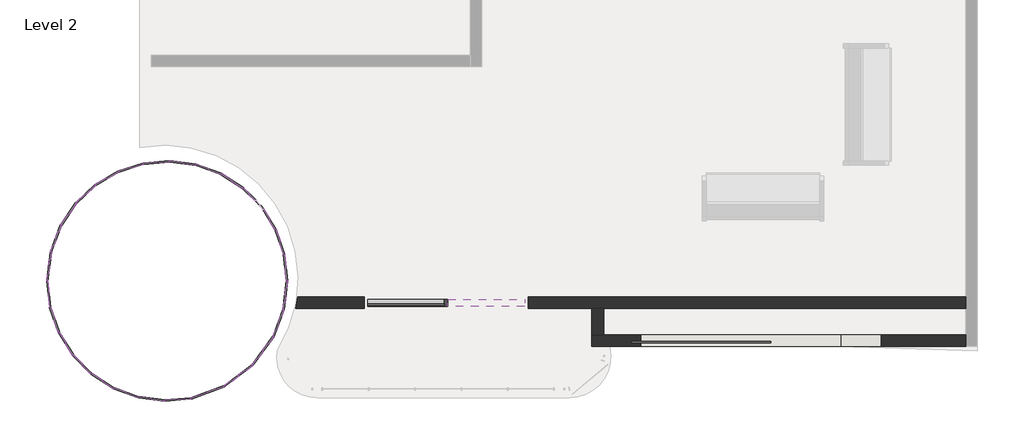
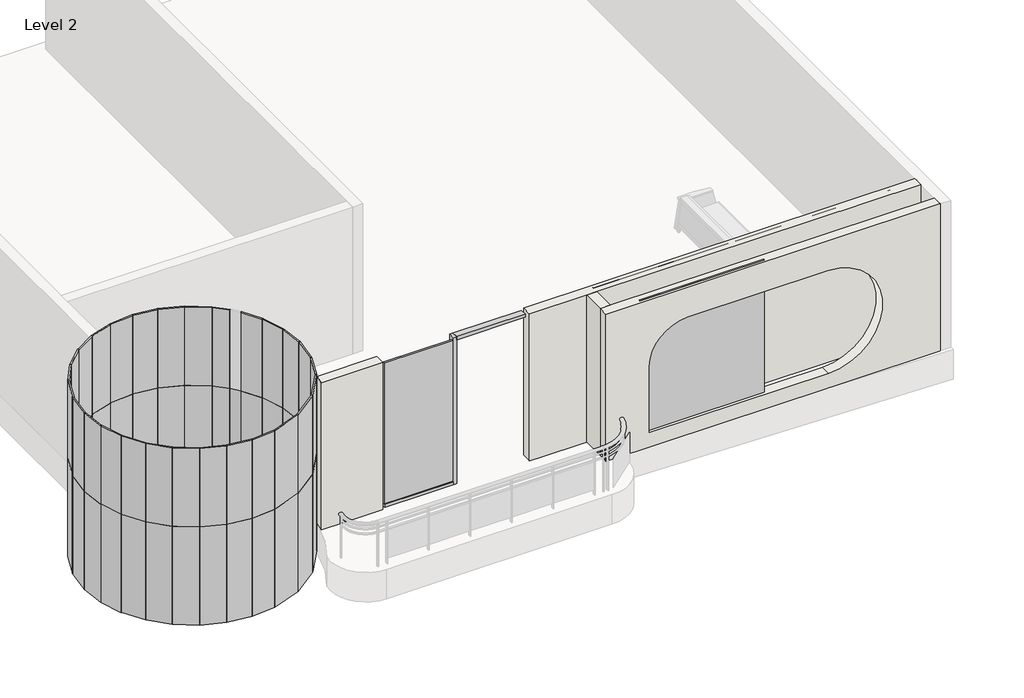
# One storey, part 1 of 2: 58 plates, 4 walls, 3 members.
"""IFC4 building model written with IfcOpenShell, lengths in millimetres."""

from ifc_helpers import new_model, si_unit, point, frame, frame_2d, origin, place, context, project, spatial, polyline, circle_curve, trimmed, segment, composite_curve, outline, extrude, faceted_brep, transform, mapped, element, save
from ifc_brep_helpers import plane_surface, revolved_surface, advanced_brep
from components import member_eaba9652, member_0c868e12, system_panel_glazed_f1c144f9, system_panel_glazed_8ed2b2ee, system_panel_glazed_c7815b78, system_panel_glazed_220ba5f3, system_panel_glazed_11fb153e, system_panel_glazed_2f540b85, system_panel_glazed_4848e608, system_panel_glazed_8b35a0ff, system_panel_glazed_6d1bb68c, system_panel_glazed_cb3ffd69, system_panel_glazed_404d015f, system_panel_glazed_7b556abe, system_panel_glazed_c60cfc80, system_panel_glazed_8d480110

model = new_model("IFC4")

# Units and contexts
model_context = context("Model", 3, world=origin())
ifc_project = project(units=[si_unit("LENGTHUNIT", "METRE", prefix="MILLI")], contexts=[model_context])

# Site, building, storey
site = spatial("IfcSite", under=ifc_project)
building = spatial("IfcBuilding", under=site)
storey = spatial("IfcBuildingStorey", under=building, Name="Level 2", Elevation=3048.0)

# Members
placement = place(None, origin())
member_shape = member_eaba9652(model_context)
element("IfcMember", 1, ObjectType="Rectangular Mullion : 2.5\" x 5\" rectangular", at=placement, inside=storey, context=model_context, shape_type="MappedRepresentation", body=[
    mapped(member_shape, transform((-7672.5789001, -1482.8937024, 3657.6), x_axis=(-1.0, 0.0, 0.0), y_axis=(0.0, 1.0, 0.0), z_axis=(0.0, 0.0, -1.0))),
])
member_2_shape = member_0c868e12(model_context)
element("IfcMember", 2, ObjectType="Rectangular Mullion : 2.5\" x 5\" rectangular", at=placement, inside=storey, context=model_context, shape_type="MappedRepresentation", body=[
    mapped(member_2_shape, transform((-7640.8289001, -1482.8937024, 6705.6), x_axis=(0.0, 0.0, 1.0), y_axis=(0.0, 1.0, 0.0), z_axis=(-1.0, 0.0, 0.0))),
])
element("IfcMember", 3, ObjectType="Rectangular Mullion : 2.5\" x 5\" rectangular", at=placement, inside=storey, context=model_context, shape_type="MappedRepresentation", body=[
    mapped(member_2_shape, transform((-7704.3289001, -1482.8937024, 3657.6), x_axis=(0.0, 0.0, -1.0), y_axis=(0.0, 1.0, 0.0), z_axis=(1.0, 0.0, 0.0))),
])

# Plates
system_panel_glazed_shape = system_panel_glazed_f1c144f9(model_context)
element("IfcPlate", 4, ObjectType="System Panel : Glazed", at=placement, inside=storey, context=model_context, shape_type="MappedRepresentation", body=[
    mapped(system_panel_glazed_shape, transform((-14541.9245022, -346.5978939, 3657.6), x_axis=(-0.3551689475306269, -0.9348021281051873, 0.0), y_axis=(0.9348021281051873, -0.3551689475306269, 0.0), z_axis=(0.0, 0.0, 1.0))),
])
element("IfcPlate", 5, ObjectType="System Panel : Glazed", at=placement, inside=storey, context=model_context, shape_type="MappedRepresentation", body=[
    mapped(system_panel_glazed_shape, transform((-10582.1178502, -1851.0877948, 3657.6), x_axis=(0.35516894753064066, 0.934802128105182, 0.0), y_axis=(-0.934802128105182, 0.35516894753064066, 0.0), z_axis=(0.0, 0.0, 1.0))),
])
element("IfcPlate", 6, ObjectType="System Panel : Glazed", at=placement, inside=storey, context=model_context, shape_type="MappedRepresentation", body=[
    mapped(system_panel_glazed_shape, transform((-10459.5232171, -1354.5613954, 3657.6), x_axis=(0.12073632210407238, 0.9926846128175765, 0.0), y_axis=(-0.9926846128175765, 0.12073632210407238, 0.0), z_axis=(0.0, 0.0, 1.0))),
])
element("IfcPlate", 7, ObjectType="System Panel : Glazed", at=placement, inside=storey, context=model_context, shape_type="MappedRepresentation", body=[
    mapped(system_panel_glazed_shape, transform((-14664.5191354, -843.1242933, 3657.6), x_axis=(-0.12073632210406242, -0.9926846128175777, 0.0), y_axis=(0.9926846128175777, -0.12073632210406242, 0.0), z_axis=(0.0, 0.0, 1.0))),
])
system_panel_glazed_2_shape = system_panel_glazed_8ed2b2ee(model_context)
element("IfcPlate", 8, ObjectType="System Panel : Glazed", at=placement, inside=storey, context=model_context, shape_type="MappedRepresentation", body=[
    mapped(system_panel_glazed_2_shape, transform((-11841.3777431, -3082.3793017, 3657.6), x_axis=(0.9398911711666007, 0.34147413718036645, 0.0), y_axis=(-0.34147413718036645, 0.9398911711666007, 0.0), z_axis=(0.0, 0.0, 1.0))),
])
element("IfcPlate", 9, ObjectType="System Panel : Glazed", at=placement, inside=storey, context=model_context, shape_type="MappedRepresentation", body=[
    mapped(system_panel_glazed_2_shape, transform((-10858.9635423, -2345.1728692, 3657.6), x_axis=(0.5905687200141164, 0.8069873524045393, 0.0), y_axis=(-0.8069873524045393, 0.5905687200141164, 0.0), z_axis=(0.0, 0.0, 1.0))),
])
element("IfcPlate", 10, ObjectType="System Panel : Glazed", at=placement, inside=storey, context=model_context, shape_type="MappedRepresentation", body=[
    mapped(system_panel_glazed_2_shape, transform((-11295.3522982, -2786.8279712, 3657.6), x_axis=(0.7998453025525061, 0.6002062078858317, 0.0), y_axis=(-0.6002062078858317, 0.7998453025525061, 0.0), z_axis=(0.0, 0.0, 1.0))),
])
system_panel_glazed_3_shape = system_panel_glazed_c7815b78(model_context)
element("IfcPlate", 11, ObjectType="System Panel : Glazed", at=placement, inside=storey, context=model_context, shape_type="MappedRepresentation", body=[
    mapped(system_panel_glazed_3_shape, transform((-10454.4737362, -864.5204039, 3657.6), x_axis=(-0.11050163420416613, 0.993875942378227, 0.0), y_axis=(-0.993875942378227, -0.11050163420416613, 0.0), z_axis=(0.0, 0.0, 1.0))),
])
element("IfcPlate", 12, ObjectType="System Panel : Glazed", at=placement, inside=storey, context=model_context, shape_type="MappedRepresentation", body=[
    mapped(system_panel_glazed_3_shape, transform((-14669.5686163, -1333.1652848, 3657.6), x_axis=(0.11050163420415138, -0.9938759423782286, 0.0), y_axis=(0.9938759423782286, 0.11050163420415138, 0.0), z_axis=(0.0, 0.0, 1.0))),
])
element("IfcPlate", 13, ObjectType="System Panel : Glazed", at=placement, inside=storey, context=model_context, shape_type="MappedRepresentation", body=[
    mapped(system_panel_glazed_3_shape, transform((-11410.1424167, 681.5611944, 3657.6), x_axis=(-0.8396018558176894, 0.5432022861766066, 0.0), y_axis=(-0.5432022861766066, -0.8396018558176894, 0.0), z_axis=(0.0, 0.0, 1.0))),
])
element("IfcPlate", 14, ObjectType="System Panel : Glazed", at=placement, inside=storey, context=model_context, shape_type="MappedRepresentation", body=[
    mapped(system_panel_glazed_3_shape, transform((-13212.0893695, 919.590846, 3657.6), x_axis=(-0.9518517343814786, -0.3065587639506839, 0.0), y_axis=(0.3065587639506839, -0.9518517343814786, 0.0), z_axis=(0.0, 0.0, 1.0))),
])
element("IfcPlate", 15, ObjectType="System Panel : Glazed", at=placement, inside=storey, context=model_context, shape_type="MappedRepresentation", body=[
    mapped(system_panel_glazed_3_shape, transform((-12839.7224363, -3201.1142893, 3657.6), x_axis=(0.9913878918151698, -0.1309581916577702, 0.0), y_axis=(0.1309581916577702, 0.9913878918151698, 0.0), z_axis=(0.0, 0.0, 1.0))),
])
element("IfcPlate", 16, ObjectType="System Panel : Glazed", at=placement, inside=storey, context=model_context, shape_type="MappedRepresentation", body=[
    mapped(system_panel_glazed_3_shape, transform((-14365.783041, -2213.7896382, 3657.6), x_axis=(0.5257859322352114, -0.8506169252157811, 0.0), y_axis=(0.8506169252157811, 0.5257859322352114, 0.0), z_axis=(0.0, 0.0, 1.0))),
])
element("IfcPlate", 17, ObjectType="System Panel : Glazed", at=placement, inside=storey, context=model_context, shape_type="MappedRepresentation", body=[
    mapped(system_panel_glazed_3_shape, transform((-13713.8999358, -2879.2468831, 3657.6), x_axis=(0.8396018558176805, -0.5432022861766201, 0.0), y_axis=(0.5432022861766201, 0.8396018558176805, 0.0), z_axis=(0.0, 0.0, 1.0))),
])
element("IfcPlate", 18, ObjectType="System Panel : Glazed", at=placement, inside=storey, context=model_context, shape_type="MappedRepresentation", body=[
    mapped(system_panel_glazed_3_shape, transform((-14014.4059364, 446.2272921, 3657.6), x_axis=(-0.7286232370002992, -0.6849147235263715, 0.0), y_axis=(0.6849147235263715, -0.7286232370002992, 0.0), z_axis=(0.0, 0.0, 1.0))),
])
element("IfcPlate", 19, ObjectType="System Panel : Glazed", at=placement, inside=storey, context=model_context, shape_type="MappedRepresentation", body=[
    mapped(system_panel_glazed_3_shape, transform((-12284.3199161, 1003.4286006, 3657.6), x_axis=(-0.9913878918151723, 0.1309581916577514, 0.0), y_axis=(-0.1309581916577514, -0.9913878918151723, 0.0), z_axis=(0.0, 0.0, 1.0))),
])
element("IfcPlate", 20, ObjectType="System Panel : Glazed", at=placement, inside=storey, context=model_context, shape_type="MappedRepresentation", body=[
    mapped(system_panel_glazed_3_shape, transform((-12752.8652893, 1013.0855973, 3657.6), x_axis=(-0.9959419324521102, -0.08999815100076568, 0.0), y_axis=(0.08999815100076568, -0.9959419324521102, 0.0), z_axis=(0.0, 0.0, 1.0))),
])
element("IfcPlate", 21, ObjectType="System Panel : Glazed", at=placement, inside=storey, context=model_context, shape_type="MappedRepresentation", body=[
    mapped(system_panel_glazed_3_shape, transform((-11829.3381514, 891.0915272, 3657.6), x_axis=(-0.9384120429483949, 0.34551821608913763, 0.0), y_axis=(-0.34551821608913763, -0.9384120429483949, 0.0), z_axis=(0.0, 0.0, 1.0))),
])
element("IfcPlate", 22, ObjectType="System Panel : Glazed", at=placement, inside=storey, context=model_context, shape_type="MappedRepresentation", body=[
    mapped(system_panel_glazed_3_shape, transform((-10557.4115054, -407.3204039, 3657.6), x_axis=(-0.3261077326604367, 0.9453326116764772, 0.0), y_axis=(-0.9453326116764772, -0.3261077326604367, 0.0), z_axis=(0.0, 0.0, 1.0))),
])
element("IfcPlate", 23, ObjectType="System Panel : Glazed", at=placement, inside=storey, context=model_context, shape_type="MappedRepresentation", body=[
    mapped(system_panel_glazed_3_shape, transform((-12371.1770631, -3210.771286, 3657.6), x_axis=(0.9959419324521115, 0.08999815100075, 0.0), y_axis=(-0.08999815100075, 0.9959419324521115, 0.0), z_axis=(0.0, 0.0, 1.0))),
])
element("IfcPlate", 24, ObjectType="System Panel : Glazed", at=placement, inside=storey, context=model_context, shape_type="MappedRepresentation", body=[
    mapped(system_panel_glazed_3_shape, transform((-13294.7042011, -3088.7772159, 3657.6), x_axis=(0.9384120429483891, -0.34551821608915334, 0.0), y_axis=(0.34551821608915334, 0.9384120429483891, 0.0), z_axis=(0.0, 0.0, 1.0))),
])
element("IfcPlate", 25, ObjectType="System Panel : Glazed", at=placement, inside=storey, context=model_context, shape_type="MappedRepresentation", body=[
    mapped(system_panel_glazed_3_shape, transform((-14076.8350959, -2582.7572647, 3657.6), x_axis=(0.6997834615185511, -0.7143550286692988, 0.0), y_axis=(0.7143550286692988, 0.6997834615185511, 0.0), z_axis=(0.0, 0.0, 1.0))),
])
element("IfcPlate", 26, ObjectType="System Panel : Glazed", at=placement, inside=storey, context=model_context, shape_type="MappedRepresentation", body=[
    mapped(system_panel_glazed_3_shape, transform((-14566.6308471, -1790.3652848, 3657.6), x_axis=(0.32610773266042153, -0.9453326116764824, 0.0), y_axis=(0.9453326116764824, 0.32610773266042153, 0.0), z_axis=(0.0, 0.0, 1.0))),
])
element("IfcPlate", 27, ObjectType="System Panel : Glazed", at=placement, inside=storey, context=model_context, shape_type="MappedRepresentation", body=[
    mapped(system_panel_glazed_3_shape, transform((-14318.3113206, 89.4787227, 3657.6), x_axis=(-0.5603879632167612, -0.8282302401396425, 0.0), y_axis=(0.8282302401396425, -0.5603879632167612, 0.0), z_axis=(0.0, 0.0, 1.0))),
])
element("IfcPlate", 28, ObjectType="System Panel : Glazed", at=placement, inside=storey, context=model_context, shape_type="MappedRepresentation", body=[
    mapped(system_panel_glazed_3_shape, transform((-13639.5625299, 727.5108588, 3657.6), x_axis=(-0.8612707706620223, -0.508146297441245, 0.0), y_axis=(0.508146297441245, -0.8612707706620223, 0.0), z_axis=(0.0, 0.0, 1.0))),
])
system_panel_glazed_4_shape = system_panel_glazed_220ba5f3(model_context)
element("IfcPlate", 29, ObjectType="System Panel : Glazed", at=placement, inside=storey, context=model_context, shape_type="MappedRepresentation", body=[
    mapped(system_panel_glazed_4_shape, transform((-10742.3305673, -4.7597883, 3657.6), x_axis=(-0.5152811917631037, 0.8570211744263939, 0.0), y_axis=(-0.8570211744263939, -0.5152811917631037, 0.0), z_axis=(0.0, 0.0, 1.0))),
])
system_panel_glazed_5_shape = system_panel_glazed_11fb153e(model_context)
element("IfcPlate", 30, ObjectType="System Panel : Glazed", at=placement, inside=storey, context=model_context, shape_type="MappedRepresentation", body=[
    mapped(system_panel_glazed_5_shape, transform((-11098.0043985, 445.2241463, 3657.6), x_axis=(-0.7256671855033587, 0.6880458821064435, 0.0), y_axis=(-0.6880458821064435, -0.7256671855033587, 0.0), z_axis=(0.0, 0.0, 1.0))),
])
system_panel_glazed_6_shape = system_panel_glazed_2f540b85(model_context)
element("IfcPlate", 31, ObjectType="System Panel : Glazed", at=placement, inside=storey, context=model_context, shape_type="MappedRepresentation", body=[
    mapped(system_panel_glazed_6_shape, transform((-10917.0903061, 255.9395759, 3657.6), x_axis=(-0.6357445726375757, 0.7718995001694627, 0.0), y_axis=(-0.7718995001694627, -0.6357445726375757, 0.0), z_axis=(0.0, 0.0, 1.0))),
])
system_panel_glazed_7_shape = system_panel_glazed_4848e608(model_context)
element("IfcPlate", 32, ObjectType="System Panel : Glazed", at=placement, inside=storey, context=model_context, shape_type="MappedRepresentation", body=[
    mapped(system_panel_glazed_7_shape, transform((-14669.5686163, -1333.1652848, 5689.6), x_axis=(0.11050163420415138, -0.9938759423782286, 0.0), y_axis=(0.9938759423782286, 0.11050163420415138, 0.0), z_axis=(0.0, 0.0, 1.0))),
])
element("IfcPlate", 33, ObjectType="System Panel : Glazed", at=placement, inside=storey, context=model_context, shape_type="MappedRepresentation", body=[
    mapped(system_panel_glazed_7_shape, transform((-14365.783041, -2213.7896382, 5689.6), x_axis=(0.5257859322352114, -0.8506169252157811, 0.0), y_axis=(0.8506169252157811, 0.5257859322352114, 0.0), z_axis=(0.0, 0.0, 1.0))),
])
element("IfcPlate", 34, ObjectType="System Panel : Glazed", at=placement, inside=storey, context=model_context, shape_type="MappedRepresentation", body=[
    mapped(system_panel_glazed_7_shape, transform((-13713.8999358, -2879.2468831, 5689.6), x_axis=(0.8396018558176805, -0.5432022861766201, 0.0), y_axis=(0.5432022861766201, 0.8396018558176805, 0.0), z_axis=(0.0, 0.0, 1.0))),
])
element("IfcPlate", 35, ObjectType="System Panel : Glazed", at=placement, inside=storey, context=model_context, shape_type="MappedRepresentation", body=[
    mapped(system_panel_glazed_7_shape, transform((-12839.7224363, -3201.1142893, 5689.6), x_axis=(0.9913878918151698, -0.13095819165777017, 0.0), y_axis=(0.13095819165777017, 0.9913878918151698, 0.0), z_axis=(0.0, 0.0, 1.0))),
])
element("IfcPlate", 36, ObjectType="System Panel : Glazed", at=placement, inside=storey, context=model_context, shape_type="MappedRepresentation", body=[
    mapped(system_panel_glazed_7_shape, transform((-12371.1770631, -3210.771286, 5689.6), x_axis=(0.9959419324521115, 0.08999815100075002, 0.0), y_axis=(-0.08999815100075002, 0.9959419324521115, 0.0), z_axis=(0.0, 0.0, 1.0))),
])
element("IfcPlate", 37, ObjectType="System Panel : Glazed", at=placement, inside=storey, context=model_context, shape_type="MappedRepresentation", body=[
    mapped(system_panel_glazed_7_shape, transform((-13294.7042011, -3088.7772159, 5689.6), x_axis=(0.9384120429483891, -0.34551821608915334, 0.0), y_axis=(0.34551821608915334, 0.9384120429483891, 0.0), z_axis=(0.0, 0.0, 1.0))),
])
element("IfcPlate", 38, ObjectType="System Panel : Glazed", at=placement, inside=storey, context=model_context, shape_type="MappedRepresentation", body=[
    mapped(system_panel_glazed_7_shape, transform((-14076.8350959, -2582.7572647, 5689.6), x_axis=(0.6997834615185511, -0.7143550286692988, 0.0), y_axis=(0.7143550286692988, 0.6997834615185511, 0.0), z_axis=(0.0, 0.0, 1.0))),
])
element("IfcPlate", 39, ObjectType="System Panel : Glazed", at=placement, inside=storey, context=model_context, shape_type="MappedRepresentation", body=[
    mapped(system_panel_glazed_7_shape, transform((-14566.6308471, -1790.3652848, 5689.6), x_axis=(0.32610773266042153, -0.9453326116764824, 0.0), y_axis=(0.9453326116764824, 0.32610773266042153, 0.0), z_axis=(0.0, 0.0, 1.0))),
])
element("IfcPlate", 40, ObjectType="System Panel : Glazed", at=placement, inside=storey, context=model_context, shape_type="MappedRepresentation", body=[
    mapped(system_panel_glazed_7_shape, transform((-10454.4737362, -864.5204039, 5689.6), x_axis=(-0.11050163420416614, 0.993875942378227, 0.0), y_axis=(-0.993875942378227, -0.11050163420416614, 0.0), z_axis=(0.0, 0.0, 1.0))),
])
element("IfcPlate", 41, ObjectType="System Panel : Glazed", at=placement, inside=storey, context=model_context, shape_type="MappedRepresentation", body=[
    mapped(system_panel_glazed_7_shape, transform((-10557.4115054, -407.3204039, 5689.6), x_axis=(-0.32610773266043674, 0.9453326116764772, 0.0), y_axis=(-0.9453326116764772, -0.32610773266043674, 0.0), z_axis=(0.0, 0.0, 1.0))),
])
element("IfcPlate", 42, ObjectType="System Panel : Glazed", at=placement, inside=storey, context=model_context, shape_type="MappedRepresentation", body=[
    mapped(system_panel_glazed_7_shape, transform((-11410.1424167, 681.5611944, 5689.6), x_axis=(-0.8396018558176894, 0.5432022861766066, 0.0), y_axis=(-0.5432022861766066, -0.8396018558176894, 0.0), z_axis=(0.0, 0.0, 1.0))),
])
element("IfcPlate", 43, ObjectType="System Panel : Glazed", at=placement, inside=storey, context=model_context, shape_type="MappedRepresentation", body=[
    mapped(system_panel_glazed_7_shape, transform((-11829.3381514, 891.0915272, 5689.6), x_axis=(-0.9384120429483949, 0.34551821608913763, 0.0), y_axis=(-0.34551821608913763, -0.9384120429483949, 0.0), z_axis=(0.0, 0.0, 1.0))),
])
element("IfcPlate", 44, ObjectType="System Panel : Glazed", at=placement, inside=storey, context=model_context, shape_type="MappedRepresentation", body=[
    mapped(system_panel_glazed_7_shape, transform((-12284.3199161, 1003.4286006, 5689.6), x_axis=(-0.9913878918151723, 0.13095819165775144, 0.0), y_axis=(-0.13095819165775144, -0.9913878918151723, 0.0), z_axis=(0.0, 0.0, 1.0))),
])
element("IfcPlate", 45, ObjectType="System Panel : Glazed", at=placement, inside=storey, context=model_context, shape_type="MappedRepresentation", body=[
    mapped(system_panel_glazed_7_shape, transform((-12752.8652893, 1013.0855973, 5689.6), x_axis=(-0.9959419324521102, -0.08999815100076569, 0.0), y_axis=(0.08999815100076569, -0.9959419324521102, 0.0), z_axis=(0.0, 0.0, 1.0))),
])
element("IfcPlate", 46, ObjectType="System Panel : Glazed", at=placement, inside=storey, context=model_context, shape_type="MappedRepresentation", body=[
    mapped(system_panel_glazed_7_shape, transform((-13212.0893695, 919.590846, 5689.6), x_axis=(-0.9518517343814786, -0.3065587639506839, 0.0), y_axis=(0.3065587639506839, -0.9518517343814786, 0.0), z_axis=(0.0, 0.0, 1.0))),
])
element("IfcPlate", 47, ObjectType="System Panel : Glazed", at=placement, inside=storey, context=model_context, shape_type="MappedRepresentation", body=[
    mapped(system_panel_glazed_7_shape, transform((-13639.5625299, 727.5108588, 5689.6), x_axis=(-0.8612707706620224, -0.5081462974412448, 0.0), y_axis=(0.5081462974412448, -0.8612707706620224, 0.0), z_axis=(0.0, 0.0, 1.0))),
])
element("IfcPlate", 48, ObjectType="System Panel : Glazed", at=placement, inside=storey, context=model_context, shape_type="MappedRepresentation", body=[
    mapped(system_panel_glazed_7_shape, transform((-14014.4059364, 446.2272921, 5689.6), x_axis=(-0.7286232370002992, -0.6849147235263715, 0.0), y_axis=(0.6849147235263715, -0.7286232370002992, 0.0), z_axis=(0.0, 0.0, 1.0))),
])
element("IfcPlate", 49, ObjectType="System Panel : Glazed", at=placement, inside=storey, context=model_context, shape_type="MappedRepresentation", body=[
    mapped(system_panel_glazed_7_shape, transform((-14318.3113206, 89.4787227, 5689.6), x_axis=(-0.5603879632167612, -0.8282302401396425, 0.0), y_axis=(0.8282302401396425, -0.5603879632167612, 0.0), z_axis=(0.0, 0.0, 1.0))),
])
system_panel_glazed_8_shape = system_panel_glazed_8b35a0ff(model_context)
element("IfcPlate", 50, ObjectType="System Panel : Glazed", at=placement, inside=storey, context=model_context, shape_type="MappedRepresentation", body=[
    mapped(system_panel_glazed_8_shape, transform((-10742.3305673, -4.7597883, 5689.6), x_axis=(-0.5152811917631037, 0.8570211744263939, 0.0), y_axis=(-0.8570211744263939, -0.5152811917631037, 0.0), z_axis=(0.0, 0.0, 1.0))),
])
system_panel_glazed_9_shape = system_panel_glazed_6d1bb68c(model_context)
element("IfcPlate", 51, ObjectType="System Panel : Glazed", at=placement, inside=storey, context=model_context, shape_type="MappedRepresentation", body=[
    mapped(system_panel_glazed_9_shape, transform((-11098.0043985, 445.2241463, 5689.6), x_axis=(-0.7256671855033587, 0.6880458821064435, 0.0), y_axis=(-0.6880458821064435, -0.7256671855033587, 0.0), z_axis=(0.0, 0.0, 1.0))),
])
system_panel_glazed_10_shape = system_panel_glazed_cb3ffd69(model_context)
element("IfcPlate", 52, ObjectType="System Panel : Glazed", at=placement, inside=storey, context=model_context, shape_type="MappedRepresentation", body=[
    mapped(system_panel_glazed_10_shape, transform((-10582.1178502, -1851.0877948, 5689.6), x_axis=(0.3551689475306406, 0.934802128105182, 0.0), y_axis=(-0.934802128105182, 0.3551689475306406, 0.0), z_axis=(0.0, 0.0, 1.0))),
])
element("IfcPlate", 53, ObjectType="System Panel : Glazed", at=placement, inside=storey, context=model_context, shape_type="MappedRepresentation", body=[
    mapped(system_panel_glazed_10_shape, transform((-10459.5232171, -1354.5613954, 5689.6), x_axis=(0.12073632210407237, 0.9926846128175765, 0.0), y_axis=(-0.9926846128175765, 0.12073632210407237, 0.0), z_axis=(0.0, 0.0, 1.0))),
])
element("IfcPlate", 54, ObjectType="System Panel : Glazed", at=placement, inside=storey, context=model_context, shape_type="MappedRepresentation", body=[
    mapped(system_panel_glazed_10_shape, transform((-14541.9245022, -346.5978939, 5689.6), x_axis=(-0.35516894753062683, -0.9348021281051873, 0.0), y_axis=(0.9348021281051873, -0.35516894753062683, 0.0), z_axis=(0.0, 0.0, 1.0))),
])
element("IfcPlate", 55, ObjectType="System Panel : Glazed", at=placement, inside=storey, context=model_context, shape_type="MappedRepresentation", body=[
    mapped(system_panel_glazed_10_shape, transform((-14664.5191354, -843.1242933, 5689.6), x_axis=(-0.12073632210406242, -0.9926846128175777, 0.0), y_axis=(0.9926846128175777, -0.12073632210406242, 0.0), z_axis=(0.0, 0.0, 1.0))),
])
system_panel_glazed_11_shape = system_panel_glazed_404d015f(model_context)
element("IfcPlate", 56, ObjectType="System Panel : Glazed", at=placement, inside=storey, context=model_context, shape_type="MappedRepresentation", body=[
    mapped(system_panel_glazed_11_shape, transform((-11841.3777431, -3082.3793017, 5689.6), x_axis=(0.9398911711666007, 0.34147413718036645, 0.0), y_axis=(-0.34147413718036645, 0.9398911711666007, 0.0), z_axis=(0.0, 0.0, 1.0))),
])
element("IfcPlate", 57, ObjectType="System Panel : Glazed", at=placement, inside=storey, context=model_context, shape_type="MappedRepresentation", body=[
    mapped(system_panel_glazed_11_shape, transform((-10858.9635423, -2345.1728692, 5689.6), x_axis=(0.5905687200141164, 0.8069873524045393, 0.0), y_axis=(-0.8069873524045393, 0.5905687200141164, 0.0), z_axis=(0.0, 0.0, 1.0))),
])
element("IfcPlate", 58, ObjectType="System Panel : Glazed", at=placement, inside=storey, context=model_context, shape_type="MappedRepresentation", body=[
    mapped(system_panel_glazed_11_shape, transform((-11295.3522982, -2786.8279712, 5689.6), x_axis=(0.7998453025525061, 0.6002062078858317, 0.0), y_axis=(-0.6002062078858317, 0.7998453025525061, 0.0), z_axis=(0.0, 0.0, 1.0))),
])
system_panel_glazed_12_shape = system_panel_glazed_7b556abe(model_context)
element("IfcPlate", 59, ObjectType="System Panel : Glazed", at=placement, inside=storey, context=model_context, shape_type="MappedRepresentation", body=[
    mapped(system_panel_glazed_12_shape, transform((-8376.2702257, -1482.8937024, 3721.1), x_axis=(-1.0, 0.0, 0.0), y_axis=(0.0, -1.0, 0.0), z_axis=(0.0, 0.0, 1.0))),
])
system_panel_glazed_13_shape = system_panel_glazed_c60cfc80(model_context)
element("IfcPlate", 60, ObjectType="System Panel : Glazed", at=placement, inside=storey, context=model_context, shape_type="MappedRepresentation", body=[
    mapped(system_panel_glazed_13_shape, transform((-3198.1462491, -2143.2937024, 3657.6), x_axis=(-1.0, 0.0, 0.0), y_axis=(0.0, -1.0, 0.0), z_axis=(0.0, 0.0, 1.0))),
])
system_panel_glazed_14_shape = system_panel_glazed_8d480110(model_context)
element("IfcPlate", 61, ObjectType="System Panel : Glazed", at=placement, inside=storey, context=model_context, shape_type="MappedRepresentation", body=[
    mapped(system_panel_glazed_14_shape, transform((-1737.6462491, -1482.8937024, 3657.6), x_axis=(1.0, 0.0, 0.0), y_axis=(0.0, 1.0, 0.0), z_axis=(0.0, 0.0, 1.0))),
])

# Walls
element("IfcWall", 62, ObjectType="Generic - 8\"", at=placement, inside=storey, context=model_context, shape_type="SweptSolid", body=[
    extrude(outline(composite_curve([segment(polyline([(-9111.7115512, -1584.4937024), (-10312.8376694, -1584.4937024)]), True, "CONTINUOUS"), segment(trimmed(circle_curve(frame_2d((-12612.6150686, -1075.1054509)), 2355.5153315), [point((-10312.8376694, -1584.4937024))], [point((-10277.0848865, -1381.2937024))], True, "CARTESIAN"), True, "CONTINUOUS"), segment(polyline([(-10277.0848865, -1381.2937024), (-9111.7115512, -1381.2937024), (-9111.7115512, -1584.4937024)]), True, "CONTINUOUS")], self_intersect=False)), frame((0.0, 0.0, 3657.6), z_axis=(0.0, 0.0, 1.0), x_axis=(1.0, 0.0, 0.0)), (0.0, 0.0, 1.0), 3048.0),
])
element("IfcWall", 63, ObjectType="Generic - 8\"", at=placement, inside=storey, context=model_context, shape_type="AdvancedBrep", body=[
    advanced_brep(
    [(1437.3537509, -2041.6937024, 3657.6), (-4912.6462491, -2041.6937024, 3657.6), (-5115.8462491, -2041.6937024, 3657.6), (-5115.8462491, -2041.6937024, 6705.6), (-4912.6462491, -2041.6937024, 6705.6), (1437.3537509, -2041.6937024, 6705.6), (-4264.9683746, -2041.6937024, 5334.0), (-4264.9683746, -2041.6937024, 3962.4), (-759.7683746, -2041.6937024, 3962.4), (-759.7683746, -2041.6937024, 6088.3415142), (-3510.6268604, -2041.6937024, 6088.3415142), (1437.3537509, -2244.8937024, 3657.6), (1437.3537509, -2244.8937024, 6705.6), (-5115.8462491, -2244.8937024, 6705.6), (-5115.8462491, -2244.8937024, 3657.6), (-4264.9683746, -2244.8937024, 5334.0), (-3510.6268604, -2244.8937024, 6088.3415142), (-759.7683746, -2244.8937024, 6088.3415142), (-759.7683746, -2244.8937024, 3962.4), (-4264.9683746, -2244.8937024, 3962.4)],
    [
        (0, 1),
        (1, 2),
        (2, 3),
        (3, 4),
        (4, 5),
        (5, 0),
        (6, 7),
        (7, 8),
        (8, 9, circle_curve(frame((-759.7683746, -2041.6937024, 5025.3707571), z_axis=(0.0, -1.0, 0.0), x_axis=(1.0, 0.0, 0.0)), 1062.9707571)),
        (9, 10),
        (10, 6, circle_curve(frame((-3510.6268604, -2041.6937024, 5334.0), z_axis=(0.0, -1.0, 0.0), x_axis=(1.0, 0.0, 0.0)), 754.3415142)),
        (11, 12),
        (12, 13),
        (13, 14),
        (14, 11),
        (15, 16, circle_curve(frame((-3510.6268604, -2244.8937024, 5334.0), z_axis=(0.0, 1.0, 0.0), x_axis=(1.0, 0.0, 0.0)), 754.3415142)),
        (16, 17),
        (17, 18, circle_curve(frame((-759.7683746, -2244.8937024, 5025.3707571), z_axis=(0.0, 1.0, 0.0), x_axis=(1.0, 0.0, 0.0)), 1062.9707571)),
        (18, 19),
        (19, 15),
        (2, 14),
        (13, 3),
        (5, 12),
        (11, 0),
        (6, 15),
        (19, 7),
        (18, 8),
        (17, 9),
        (16, 10),
    ],
    [
        plane_surface(frame((1538.9537509, -2041.6937024, 3657.6), z_axis=(0.0, 1.0, 0.0), x_axis=(-1.0, 0.0, 0.0))),
        plane_surface(frame((1538.9537509, -2244.8937024, 3657.6), z_axis=(0.0, -1.0, 0.0), x_axis=(1.0, 0.0, 0.0))),
        plane_surface(frame((-5115.8462491, -1482.8937024, 3657.6), z_axis=(-1.0, 0.0, 0.0), x_axis=(0.0, -1.0, 0.0))),
        plane_surface(frame((1437.3537509, 16068.5062976, 3657.6), z_axis=(1.0, 0.0, 0.0), x_axis=(0.0, -1.0, 0.0))),
        plane_surface(frame((1538.9537509, -2041.6937024, 3657.6), z_axis=(0.0, 0.0, -1.0), x_axis=(0.0, -1.0, 0.0))),
        plane_surface(frame((-5014.2462491, -2041.6937024, 6705.6), z_axis=(0.0, 0.0, 1.0), x_axis=(0.0, -1.0, 0.0))),
        plane_surface(frame((-4264.9683746, -2041.6937024, 5334.0), z_axis=(1.0, 0.0, 0.0), x_axis=(0.0, -1.0, 0.0))),
        plane_surface(frame((-4264.9683746, -2041.6937024, 3962.4), z_axis=(0.0, 0.0, 1.0), x_axis=(0.0, -1.0, 0.0))),
        revolved_surface(polyline([(303.2023824999999, -2244.8937024, 5025.3707571), (303.2023824999999, -2041.6937024, 5025.3707571)]), (-759.7683746, -2143.2937024, 5025.3707571), (0.0, -1.0, 0.0)),
        plane_surface(frame((-759.7683746, -2041.6937024, 6088.3415142), z_axis=(0.0, 0.0, -1.0), x_axis=(0.0, -1.0, 0.0))),
        revolved_surface(polyline([(-2756.2853462000003, -2244.8937024, 5334.0), (-2756.2853462000003, -2041.6937024, 5334.0)]), (-3510.6268604, -2143.2937024, 5334.0), (0.0, -1.0, 0.0)),
    ],
    [
        (0, [[1, 2, 3, 4, 5, 6], [7, 8, 9, 10, 11]]),
        (1, [[12, 13, 14, 15], [16, 17, 18, 19, 20]]),
        (2, [[-3, 21, -14, 22]]),
        (3, [[-6, 23, -12, 24]]),
        (4, [[-2, -1, -24, -15, -21]]),
        (5, [[-5, -4, -22, -13, -23]]),
        (6, [[-7, 25, -20, 26]]),
        (7, [[-8, -26, -19, 27]]),
        (8, [[-9, -27, -18, 28]]),
        (9, [[-10, -28, -17, 29]]),
        (10, [[-11, -29, -16, -25]]),
    ],
),
])
element("IfcWall", 64, ObjectType="Generic - 8\"", at=placement, inside=storey, context=model_context, shape_type="Brep", body=[
    faceted_brep([(-6233.4462491, -1584.4937024, 3657.6), (-5115.8462491, -1584.4937024, 3657.6), (-4912.6462491, -1584.4937024, 3657.6), (1437.3537509, -1584.4937024, 3657.6), (1437.3537509, -1584.4937024, 6705.6), (-4912.6462491, -1584.4937024, 6705.6), (-5115.8462491, -1584.4937024, 6705.6), (-6233.4462491, -1584.4937024, 6705.6), (-6233.4462491, -1381.2937024, 3657.6), (-6233.4462491, -1381.2937024, 6705.6), (1437.3537509, -1381.2937024, 6705.6), (1437.3537509, -1381.2937024, 3657.6)], [[[0, 1, 2, 3, 4, 5, 6, 7]], [[8, 9, 10, 11]], [[3, 2, 1, 0, 8, 11]], [[7, 6, 5, 4, 10, 9]], [[0, 7, 9, 8]], [[4, 3, 11, 10]]]),
])
element("IfcWall", 65, ObjectType="Generic - 8\"", at=placement, inside=storey, context=model_context, shape_type="SweptSolid", body=[
    extrude(outline(polyline([(-5115.8462491, -2041.6937024), (-5115.8462491, -1584.4937024), (-4912.6462491, -1584.4937024), (-4912.6462491, -2041.6937024), (-5115.8462491, -2041.6937024)])), frame((0.0, 0.0, 3657.6), z_axis=(0.0, 0.0, 1.0), x_axis=(1.0, 0.0, 0.0)), (0.0, 0.0, 1.0), 3048.0),
])

save(model, "model.ifc")

# Revit data of these elements
# Type "Rectangular Mullion : 2.5\" x 5\" rectangular"
#   built-in parameter 1007304 = 0.416667 (stored number, unit not read)
#   built-in parameter 1007301 = 0.104167 (stored number, unit not read)
#   built-in parameter 1007300 = 0.104167 (stored number, unit not read)
# Type "System Panel : Glazed"
#   Construction Type Id = "GSP4R"
#   Analytic Construction = "1/8 in Pilkington single glazing"
#   Visual Light Transmittance = 0.9
#   Solar Heat Gain Coefficient = 0.86
#   Heat Transfer Coefficient (U) = 1.18115 BTU/(h·ft²·°F)
# Type "Generic - 8\""
#   Assembly Code = "B2010"
#   Layers, outside or top first: 0' - 8" no material (function 1)
# Elements 1, 2, 3 (IfcMember, "Rectangular Mullion : 2.5\" x 5\" rectangular")
#   Phase Created = New Construction
#   Materials on its faces: "Iron, Ductile"
# Elements 4, 5, 6, 7, 8, 9, 10, 11, 12, 13, 14, 15, 16, 17, 18, 19, 20, 21, 22, 23, 24, 25, 26, 27, 28, 29, 30, 31, 32, 33, 34, 35, 36, 37, 38, 39, 40, 41, 42, 43, 44, 45, 46, 47, 48, 49, 50, 51, 52, 53, 54, 55, 56, 57, 58, 59, 60, 61 (IfcPlate, "System Panel : Glazed")
#   Phase Created = New Construction
#   Materials on its faces: "Glass"
# Elements 62, 63, 64, 65 (IfcWall, "Generic - 8\"")
#   built-in parameter 1001111 = 2' - 0"
#   Top Offset = 0' - 0"
#   Base Offset = 2' - 0"
#   Unconnected Height = 10' - 0"
#   wall height = 10' - 0"
#   Phase Created = New Construction
#   Base Constraint = Level 2
#   Materials on its faces: "Default Wall"
# Materials
#   "Iron, Ductile": class "Metal", colour RGB 0 0 0, transparency 0, Description = "Ductile cast iron", Cost = 0
#   "Glass": class "Glass", colour RGB 0 128 192, transparency 0.75, Description = "Soda Lime Glass", Cost = 0
#   "Default Wall": colour RGB 128 128 128, transparency 0
